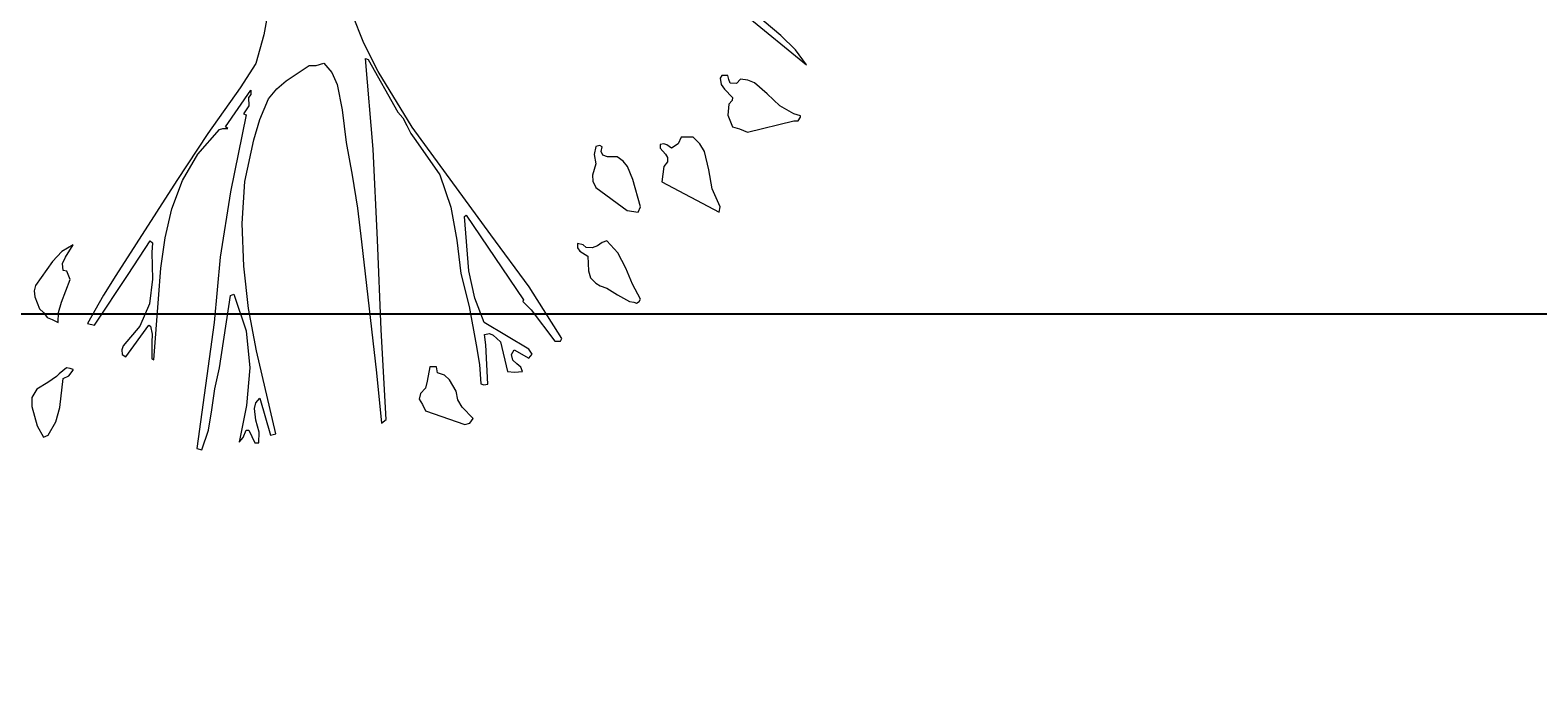
# Model space of a CAD drawing. Units: inches. Extents: x 84 to 1044, y -280 to 906.
# Tile 17 of 105: x 659 to 700, y -132 to -114. Entities that reach past the tile are written whole.
import ezdxf

# ---------------------------------------------------------------- set-up
doc = ezdxf.new("R2010")
doc.units = ezdxf.units.IN
for name, color, linetype, lineweight in [('A-ANNO-DIMS', 2, 'Continuous', 18), ('C-PROP', 7, 'Continuous', 25), ('L-PLNT', 114, 'Continuous', 15)]:
    doc.layers.add(name, color=color, linetype=linetype, lineweight=lineweight)
doc.styles.get("Standard").update_dxf_attribs({"font": 'arial.ttf'})
doc.dimstyles.get("Standard").update_dxf_attribs({"dimtxt": 0.18, "dimasz": 0.18, "dimexe": 0.18, "dimexo": 0.0625, "dimgap": 0.09, "dimtad": 0, "dimtih": 1, "dimtoh": 1, "dimdec": 4, "dimzin": 0, "dimdsep": 46, "dimtxsty": 'Standard', "dimcen": 0.09, "dimadec": 0, "dimazin": 0, "dimtfac": 1, "dimtdec": 4, "dimtofl": 0, "dimtmove": 0, "dimatfit": 3, "dimfxl": 1, "dimtolj": 1, "dimtzin": 0, "dimarcsym": 0})

# ---------------------------------------------------------------- blocks, each defined once
blk = doc.blocks.new('A$C37E508DF')
for p, q in [((0.0905, 0.4515), (0.1269, 0.482)), ((0.6483, 0.4845), (0.6539, 0.4524)), ((0.1282, 0.4734), (0.0626, 0.4198)), ((0.545, 0.4434), (0.5578, 0.4751)), ((0.0746, 0.4361), (0.0905, 0.4515)), ((0.6539, 0.4524), (0.6625, 0.4211)), ((0.0626, 0.4198), (0.0746, 0.4361)), ((0.5295, 0.4125), (0.545, 0.4434)), ((0.4922, 0.3516), (0.5295, 0.4125)), ((0.5403, 0.4254), (0.5081, 0.3679)), ((0.5347, 0.3276), (0.5433, 0.4266)), ((0.5433, 0.4266), (0.5403, 0.4254)), ((0.5797, 0.4112), (0.5741, 0.3983)), ((0.5887, 0.4215), (0.5797, 0.4112)), ((0.5969, 0.4189), (0.5887, 0.4215)), ((0.6046, 0.4189), (0.5969, 0.4189)), ((0.6295, 0.4022), (0.6046, 0.4189)), ((0.6625, 0.4211), (0.6796, 0.3945)), ((0.1055, 0.388), (0.1192, 0.4001)), ((0.1192, 0.4001), (0.1265, 0.4031)), ((0.1265, 0.4031), (0.1346, 0.4039)), ((0.1346, 0.4039), (0.1389, 0.3992)), ((0.1389, 0.3992), (0.1458, 0.3996)), ((0.1458, 0.3996), (0.1471, 0.4035)), ((0.1471, 0.4035), (0.1484, 0.4082)), ((0.1484, 0.4082), (0.1548, 0.4082)), ((0.1556, 0.3983), (0.1518, 0.3932)), ((0.1548, 0.4082), (0.1565, 0.4052)), ((0.1565, 0.4052), (0.1556, 0.3983)), ((0.5741, 0.3983), (0.5686, 0.3705)), ((0.6397, 0.3936), (0.6295, 0.4022)), ((0.6796, 0.3945), (0.7148, 0.3447)), ((0.0917, 0.3748), (0.1055, 0.388)), ((0.1518, 0.3932), (0.1432, 0.3842)), ((0.1432, 0.3842), (0.1436, 0.3808)), ((0.1436, 0.3808), (0.1471, 0.3769)), ((0.6487, 0.3825), (0.6397, 0.3936)), ((0.6582, 0.3602), (0.6487, 0.3825)), ((0.6959, 0.352), (0.668, 0.3919)), ((0.668, 0.3919), (0.668, 0.3872)), ((0.668, 0.3872), (0.6706, 0.3842)), ((0.6706, 0.3842), (0.6702, 0.3748)), ((0.069, 0.364), (0.0763, 0.3662)), ((0.069, 0.3627), (0.069, 0.364)), ((0.0716, 0.3585), (0.069, 0.3627)), ((0.0763, 0.3662), (0.0917, 0.3748)), ((0.1484, 0.3649), (0.1432, 0.352)), ((0.1471, 0.3769), (0.1484, 0.3649)), ((0.5025, 0.3619), (0.4982, 0.3537)), ((0.5081, 0.3679), (0.5025, 0.3619)), ((0.5686, 0.3705), (0.5643, 0.3349)), ((0.6702, 0.3748), (0.6762, 0.3662)), ((0.6762, 0.3662), (0.6732, 0.3653)), ((0.6732, 0.3653), (0.6903, 0.2813)), ((0.0763, 0.3585), (0.0716, 0.3585)), ((0.1269, 0.3464), (0.0763, 0.3585)), ((0.1355, 0.3499), (0.1269, 0.3464)), ((0.1432, 0.352), (0.1355, 0.3499)), ((0.4065, 0.2345), (0.4922, 0.3516)), ((0.4982, 0.3537), (0.4939, 0.3447)), ((0.665, 0.3379), (0.6582, 0.3602)), ((0.6933, 0.3503), (0.6959, 0.352)), ((0.6985, 0.3503), (0.6933, 0.3503)), ((0.7023, 0.349), (0.6985, 0.3503)), ((0.7259, 0.3224), (0.7023, 0.349)), ((0.1737, 0.325), (0.1788, 0.3336)), ((0.1788, 0.3336), (0.1861, 0.3409)), ((0.1861, 0.3409), (0.199, 0.3409)), ((0.199, 0.3409), (0.2024, 0.3336)), ((0.2024, 0.3336), (0.2097, 0.3289)), ((0.2097, 0.3289), (0.2148, 0.3323)), ((0.2148, 0.3323), (0.2182, 0.3336)), ((0.2221, 0.3289), (0.2161, 0.3224)), ((0.2182, 0.3336), (0.2221, 0.3327)), ((0.2221, 0.3327), (0.2221, 0.3289)), ((0.2851, 0.3302), (0.2877, 0.3319)), ((0.2864, 0.325), (0.2851, 0.3302)), ((0.2877, 0.3319), (0.292, 0.3306)), ((0.292, 0.3306), (0.2941, 0.322)), ((0.4884, 0.337), (0.4622, 0.2997)), ((0.4939, 0.3447), (0.4884, 0.337)), ((0.5643, 0.3349), (0.5578, 0.2993)), ((0.6745, 0.2924), (0.665, 0.3379)), ((0.7148, 0.3447), (0.7487, 0.2937)), ((0.1689, 0.3053), (0.1737, 0.325)), ((0.2161, 0.3224), (0.214, 0.3186)), ((0.214, 0.3186), (0.214, 0.3139)), ((0.214, 0.3139), (0.2182, 0.3087)), ((0.2577, 0.3087), (0.2624, 0.3147)), ((0.2624, 0.3147), (0.2689, 0.3194)), ((0.2689, 0.3194), (0.2796, 0.3194)), ((0.2796, 0.3194), (0.2847, 0.3211)), ((0.2847, 0.3211), (0.2864, 0.325)), ((0.2941, 0.322), (0.292, 0.3117)), ((0.53, 0.229), (0.5347, 0.3276)), ((0.7427, 0.2937), (0.7259, 0.3224)), ((0.1655, 0.2843), (0.1689, 0.3053)), ((0.2182, 0.3087), (0.2204, 0.292)), ((0.2517, 0.2946), (0.2577, 0.3087)), ((0.292, 0.3117), (0.2959, 0.2993)), ((0.2959, 0.2993), (0.2954, 0.2928)), ((0.4622, 0.2997), (0.4502, 0.2645)), ((0.5578, 0.2993), (0.5518, 0.2633)), ((0.1565, 0.265), (0.1655, 0.2843)), ((0.2204, 0.292), (0.1578, 0.259)), ((0.2436, 0.265), (0.2517, 0.2946)), ((0.292, 0.286), (0.2581, 0.2607)), ((0.2954, 0.2928), (0.292, 0.286)), ((0.6775, 0.2465), (0.6745, 0.2924)), ((0.6903, 0.2813), (0.7015, 0.2101)), ((0.7542, 0.2628), (0.7427, 0.2937)), ((0.7487, 0.2937), (0.8151, 0.1899)), ((0.1578, 0.259), (0.1565, 0.265)), ((0.2461, 0.259), (0.2436, 0.265)), ((0.4502, 0.2645), (0.4438, 0.2285)), ((0.5518, 0.2633), (0.5475, 0.2268)), ((0.2581, 0.2607), (0.2461, 0.259)), ((0.4335, 0.2556), (0.3709, 0.1634)), ((0.4305, 0.1951), (0.4352, 0.2543)), ((0.4352, 0.2543), (0.4335, 0.2556)), ((0.6758, 0.2002), (0.6775, 0.2465)), ((0.7615, 0.2311), (0.7542, 0.2628)), ((0.3649, 0.1775), (0.4065, 0.2345)), ((0.7662, 0.1981), (0.7615, 0.2311)), ((0.2594, 0.1981), (0.268, 0.2148)), ((0.268, 0.2148), (0.28, 0.2277)), ((0.28, 0.2277), (0.2851, 0.226)), ((0.2851, 0.226), (0.2903, 0.2225)), ((0.2903, 0.2225), (0.2963, 0.22)), ((0.2963, 0.22), (0.3027, 0.2204)), ((0.3096, 0.2165), (0.301, 0.211)), ((0.3027, 0.2204), (0.3061, 0.2234)), ((0.3061, 0.2234), (0.3122, 0.2247)), ((0.3122, 0.22), (0.3096, 0.2165)), ((0.3122, 0.2247), (0.3122, 0.22)), ((0.4438, 0.2285), (0.4391, 0.1921)), ((0.5261, 0.1308), (0.53, 0.229)), ((0.5475, 0.2268), (0.5313, 0.084)), ((0.7778, 0.2277), (0.7752, 0.2255)), ((0.7752, 0.2255), (0.7761, 0.2152)), ((0.7761, 0.2152), (0.7752, 0.1861)), ((0.8018, 0.1912), (0.7778, 0.2277)), ((0.8619, 0.2234), (0.8739, 0.2161)), ((0.87, 0.2101), (0.8619, 0.2234)), ((0.8739, 0.2161), (0.8841, 0.2054)), ((0.2521, 0.1805), (0.2594, 0.1981)), ((0.301, 0.211), (0.3002, 0.1951)), ((0.6706, 0.1539), (0.6758, 0.2002)), ((0.7015, 0.2101), (0.7079, 0.1389)), ((0.7688, 0.1646), (0.7662, 0.1981)), ((0.8734, 0.2032), (0.87, 0.2101)), ((0.8726, 0.1955), (0.8734, 0.2032)), ((0.8841, 0.2054), (0.9026, 0.1792)), ((0.292, 0.1818), (0.2873, 0.1788)), ((0.298, 0.1874), (0.292, 0.1818)), ((0.3002, 0.1951), (0.298, 0.1874)), ((0.4241, 0.1651), (0.4305, 0.1951)), ((0.4391, 0.1921), (0.4301, 0.1561)), ((0.7752, 0.1861), (0.7787, 0.1591)), ((0.8383, 0.1359), (0.8018, 0.1912)), ((0.8151, 0.1899), (0.8288, 0.1685)), ((0.8649, 0.1857), (0.8687, 0.1947)), ((0.8743, 0.1608), (0.8649, 0.1857)), ((0.8687, 0.1947), (0.8726, 0.1955)), ((0.2436, 0.1642), (0.2521, 0.1805)), ((0.2684, 0.1689), (0.2556, 0.1616)), ((0.28, 0.1762), (0.2684, 0.1689)), ((0.2873, 0.1788), (0.28, 0.1762)), ((0.3293, 0.1213), (0.3649, 0.1775)), ((0.4138, 0.1389), (0.4241, 0.1651)), ((0.6865, 0.1698), (0.6732, 0.1295)), ((0.6903, 0.1681), (0.6865, 0.1698)), ((0.7023, 0.0892), (0.6903, 0.1681)), ((0.774, 0.0982), (0.7688, 0.1646)), ((0.8288, 0.1685), (0.846, 0.1376)), ((0.9035, 0.1668), (0.8983, 0.1535)), ((0.9026, 0.1792), (0.9043, 0.1732)), ((0.9043, 0.1732), (0.9035, 0.1668)), ((0.2448, 0.1616), (0.2436, 0.1642)), ((0.2478, 0.1599), (0.2448, 0.1616)), ((0.2508, 0.1608), (0.2478, 0.1599)), ((0.2556, 0.1616), (0.2508, 0.1608)), ((0.3628, 0.1526), (0.337, 0.1183)), ((0.3692, 0.1591), (0.3628, 0.1526)), ((0.3718, 0.1616), (0.3692, 0.1591)), ((0.3709, 0.1634), (0.3718, 0.1616)), ((0.4301, 0.1561), (0.4224, 0.1145)), ((0.662, 0.108), (0.6706, 0.1539)), ((0.7787, 0.1591), (0.789, 0.1346)), ((0.8777, 0.1496), (0.8743, 0.1608)), ((0.8781, 0.1389), (0.8777, 0.1496)), ((0.894, 0.1496), (0.8902, 0.1441)), ((0.8983, 0.1535), (0.894, 0.1496)), ((0.3653, 0.1098), (0.4138, 0.1389)), ((0.7079, 0.1389), (0.7268, 0.0013)), ((0.7774, 0.1346), (0.7757, 0.1261)), ((0.7791, 0.1359), (0.7774, 0.1346)), ((0.8044, 0.1012), (0.7791, 0.1359)), ((0.789, 0.1346), (0.8074, 0.1132)), ((0.846, 0.1376), (0.8383, 0.1359)), ((0.8846, 0.1419), (0.8781, 0.1389)), ((0.8902, 0.1441), (0.8846, 0.1419)), ((0.3306, 0.1183), (0.3293, 0.1213)), ((0.337, 0.1183), (0.3306, 0.1183)), ((0.3962, 0.1175), (0.3885, 0.0853)), ((0.4039, 0.1248), (0.3962, 0.1175)), ((0.4082, 0.1269), (0.4039, 0.1248)), ((0.4134, 0.1256), (0.4082, 0.1269)), ((0.4121, 0.1145), (0.4134, 0.1256)), ((0.5205, 0.033), (0.5261, 0.1308)), ((0.6732, 0.1295), (0.6693, 0.0892)), ((0.7757, 0.1261), (0.7761, 0.117)), ((0.7761, 0.117), (0.7761, 0.099)), ((0.3615, 0.1042), (0.3653, 0.1098)), ((0.3653, 0.0999), (0.3615, 0.1042)), ((0.3812, 0.1089), (0.3653, 0.0999)), ((0.3842, 0.1037), (0.3812, 0.1089)), ((0.3825, 0.0978), (0.3842, 0.1037)), ((0.4099, 0.0716), (0.4121, 0.1145)), ((0.4224, 0.1145), (0.4189, 0.093)), ((0.641, 0.0172), (0.662, 0.108)), ((0.7761, 0.099), (0.774, 0.0982)), ((0.8083, 0.1037), (0.8044, 0.1012)), ((0.8074, 0.1132), (0.8087, 0.1089)), ((0.8087, 0.1089), (0.8083, 0.1037)), ((0.3722, 0.0853), (0.3739, 0.09)), ((0.3808, 0.0845), (0.3722, 0.0853)), ((0.3739, 0.09), (0.3782, 0.0935)), ((0.3782, 0.0935), (0.3825, 0.0978)), ((0.3885, 0.0853), (0.3808, 0.0845)), ((0.4189, 0.093), (0.4176, 0.072)), ((0.4571, 0.0815), (0.4648, 0.084)), ((0.4648, 0.084), (0.4657, 0.0905)), ((0.4657, 0.0905), (0.473, 0.0905)), ((0.473, 0.0905), (0.476, 0.0746)), ((0.5313, 0.084), (0.5257, 0.0291)), ((0.6693, 0.0892), (0.6728, 0.0484)), ((0.7075, 0.0665), (0.7023, 0.0892)), ((0.8619, 0.0875), (0.8649, 0.0887)), ((0.8619, 0.0866), (0.8619, 0.0875)), ((0.8666, 0.0806), (0.8619, 0.0866)), ((0.8649, 0.0887), (0.8691, 0.0892)), ((0.8691, 0.0892), (0.8769, 0.0827)), ((0.8769, 0.0827), (0.8799, 0.0797)), ((0.4142, 0.0707), (0.4099, 0.0716)), ((0.4176, 0.072), (0.4142, 0.0707)), ((0.4442, 0.0639), (0.4515, 0.0763)), ((0.4515, 0.0763), (0.4571, 0.0815)), ((0.476, 0.0746), (0.4777, 0.0673)), ((0.4777, 0.0673), (0.4832, 0.0613)), ((0.7105, 0.0437), (0.7075, 0.0665)), ((0.8726, 0.0776), (0.8666, 0.0806)), ((0.8764, 0.0459), (0.8726, 0.0776)), ((0.8799, 0.0797), (0.8893, 0.0733)), ((0.8893, 0.0733), (0.9013, 0.066)), ((0.9013, 0.066), (0.9069, 0.057)), ((0.4378, 0.0463), (0.4425, 0.0544)), ((0.4425, 0.0544), (0.4442, 0.0639)), ((0.4811, 0.0493), (0.4777, 0.0424)), ((0.4845, 0.0553), (0.4811, 0.0493)), ((0.4832, 0.0613), (0.4845, 0.0553)), ((0.6582, 0.0562), (0.6466, 0.0159)), ((0.6625, 0.051), (0.6582, 0.0562)), ((0.6642, 0.045), (0.6625, 0.051)), ((0.9069, 0.057), (0.9069, 0.0471)), ((0.4258, 0.0339), (0.4378, 0.0463)), ((0.4296, 0.0291), (0.4258, 0.0339)), ((0.4777, 0.0424), (0.4348, 0.0274)), ((0.5257, 0.0291), (0.5205, 0.033)), ((0.6625, 0.0321), (0.6642, 0.045)), ((0.6728, 0.0484), (0.6809, 0.0082)), ((0.7144, 0.0214), (0.7105, 0.0437)), ((0.8807, 0.0304), (0.8764, 0.0459)), ((0.9069, 0.0471), (0.9009, 0.0261)), ((0.4348, 0.0274), (0.4296, 0.0291)), ((0.6466, 0.0159), (0.641, 0.0172)), ((0.659, 0.0193), (0.6625, 0.0321)), ((0.6595, 0.0077), (0.659, 0.0193)), ((0.6702, 0.0214), (0.6637, 0.0077)), ((0.6732, 0.0214), (0.6702, 0.0214)), ((0.6766, 0.0133), (0.6732, 0.0214)), ((0.7216, 0), (0.7144, 0.0214)), ((0.8889, 0.0159), (0.8807, 0.0304)), ((0.9009, 0.0261), (0.894, 0.0137)), ((0.6637, 0.0077), (0.6595, 0.0077)), ((0.6809, 0.0082), (0.6766, 0.0133)), ((0.7268, 0.0013), (0.7216, 0)), ((0.894, 0.0137), (0.8889, 0.0159))]:
    blk.add_line(p, q)
blk = doc.blocks.new('*D60')
at = {"layer": 'A-ANNO-DIMS', "color": 0, "lineweight": -2, "transparency": 16777216}
for p, q in [((134.179, -121.942), (134.179, -180.64)), ((992.074, -121.942), (992.074, -180.64)), ((134.359, -180.46), (562.733, -180.46)), ((991.894, -180.46), (563.521, -180.46))]:
    blk.add_line(p, q, dxfattribs=at)
at = {"layer": 'A-ANNO-DIMS', "color": 0, "transparency": 16777216}
for points in [[(134.359, -180.43), (134.359, -180.49), (134.179, -180.46)], [(991.894, -180.43), (991.894, -180.49), (992.074, -180.46)]]:
    blk.add_solid(points, dxfattribs=at)
at = {"layer": 'Defpoints', "color": 0, "transparency": 16777216}
for p in [(134.179, -121.88), (992.074, -121.88), (992.074, -180.46)]:
    blk.add_point(p, dxfattribs=at)
at = {"layer": 'A-ANNO-DIMS', "color": 0, "transparency": 16777216, "insert": (563.127, -180.46), "char_height": 0.18, "attachment_point": 5}
blk.add_mtext('\\A1;857.9', dxfattribs=at)

msp = doc.modelspace()

# ---------------------------------------------------------------- linework, layer by layer
at = {"layer": 'C-PROP'}
msp.add_lwpolyline([(143.179, -121.88), (134.179, -121.88), (134.179, 856.12), (992.074, 856.12), (992.074, -121.88), (624.574, -121.88)], dxfattribs=at)

# ---------------------------------------------------------------- block references
at = {"layer": 'L-PLNT', "xscale": -24.64361536662419, "yscale": 24.64361536662419, "zscale": 24.64361536662419}
msp.add_blockref('A$C37E508DF', (681.765, -125.52), dxfattribs=at)

# ---------------------------------------------------------------- dimensions: what is measured, and where the dimension line sits
at = {"layer": 'A-ANNO-DIMS'}
dim = msp.add_linear_dim(base=(992.074, -180.46), p1=(134.179, -121.88), p2=(992.074, -121.88), dimstyle='Standard', override={"dimdec": 1, "dimlfac": 1, "dimrnd": 0, "dimzin": 0, "dimdsep": 46, "dimlunit": 2}, dxfattribs=at)
dim.commit()
dim.dimension.update_dxf_attribs({"geometry": '*D60', "text_midpoint": (563.127, -180.46)})

doc.saveas('drawing.dxf')
